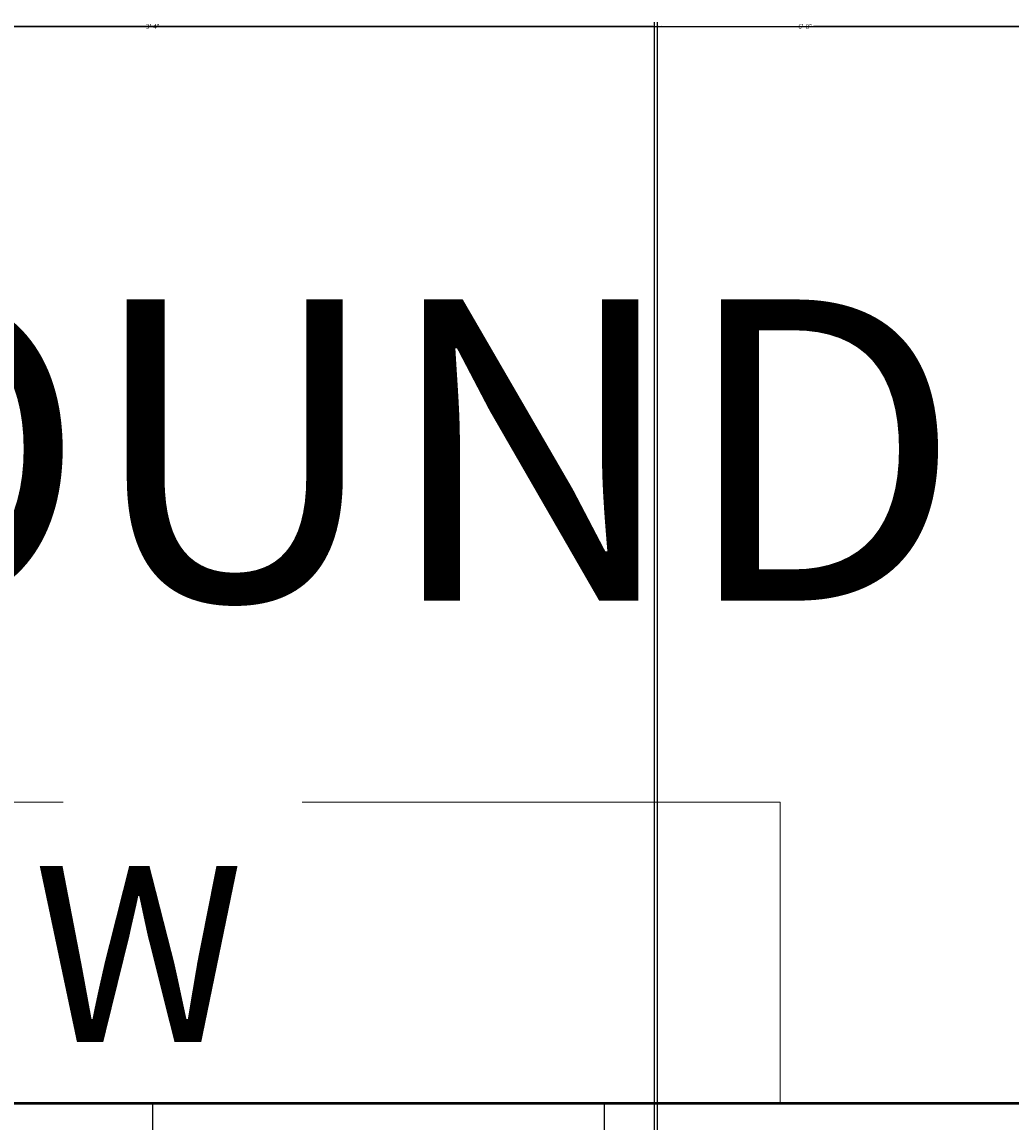
# Model space of a CAD drawing. Units: inches. Extents: x 37 to 824, y -700 to 234.
# Tile 60 of 77: x 225 to 264, y 190 to 234. Entities that reach past the tile are written whole.
import ezdxf

# ---------------------------------------------------------------- set-up
doc = ezdxf.new("R2010")
doc.units = ezdxf.units.IN
doc.header["$MEASUREMENT"] = 0
doc.linetypes.add('DASHED', pattern=[19.05, 12.7, -6.35])
for name, color, linetype, lineweight in [('A-ANNO-DIMS', 2, 'Continuous', 18), ('A-ANNO-TEXT', 7, 'Continuous', 18), ('A-GLAZ', 4, 'Continuous', 25), ('A-ROOF-OVHD', 1, 'DASHED', 18), ('A-WALL', 2, 'Continuous', 50)]:
    doc.layers.add(name, color=color, linetype=linetype, lineweight=lineweight)
doc.styles.get("Standard").update_dxf_attribs({"font": 'arial.ttf'})
doc.dimstyles.get("Standard").update_dxf_attribs({"dimtxt": 0.18, "dimasz": 0.18, "dimexe": 0.18, "dimexo": 0.0625, "dimgap": 0.09, "dimtad": 0, "dimtih": 1, "dimtoh": 1, "dimdec": 1, "dimzin": 0, "dimdsep": 46, "dimlunit": 4, "dimtxsty": 'Standard', "dimcen": 0.09, "dimadec": 0, "dimazin": 0, "dimtfac": 1, "dimtdec": 1, "dimtofl": 0, "dimtmove": 0, "dimatfit": 3, "dimfxl": 1, "dimtolj": 1, "dimtzin": 0, "dimarcsym": 0})

# ---------------------------------------------------------------- blocks, each defined once
blk = doc.blocks.new('WIN-900')
for p, q in [((0, 9), (0, 0)), ((2, 9), (2, 0)), ((20, 9), (20, 0)), ((38, 9), (38, 0)), ((40, 9), (40, 0)), ((38, 5.5), (2, 5.5)), ((38, 3.5), (2, 3.5))]:
    blk.add_line(p, q)
blk = doc.blocks.new('*D45')
at = {"layer": 'A-ANNO-DIMS', "color": 0, "lineweight": -2, "ltscale": 0.5, "transparency": 16777216}
for p, q in [((210.077, 191.153), (210.077, 234.17)), ((250.077, 191.153), (250.077, 234.17)), ((210.257, 233.99), (229.748, 233.99)), ((249.897, 233.99), (230.406, 233.99))]:
    blk.add_line(p, q, dxfattribs=at)
at = {"layer": 'A-ANNO-DIMS', "color": 0, "ltscale": 0.5, "transparency": 16777216}
for points in [[(210.257, 234.02), (210.257, 233.96), (210.077, 233.99)], [(249.897, 234.02), (249.897, 233.96), (250.077, 233.99)]]:
    blk.add_solid(points, dxfattribs=at)
at = {"layer": 'Defpoints', "color": 0, "ltscale": 0.5, "transparency": 16777216}
for p in [(250.077, 233.99), (210.077, 191.09), (250.077, 191.09)]:
    blk.add_point(p, dxfattribs=at)
at = {"layer": 'A-ANNO-DIMS', "color": 0, "ltscale": 0.5, "transparency": 16777216, "insert": (230.077, 233.99), "char_height": 0.18, "attachment_point": 5}
blk.add_mtext('\\A1;3\'-4"', dxfattribs=at)
blk = doc.blocks.new('*D46')
at = {"layer": 'A-ANNO-DIMS', "color": 0, "lineweight": -2, "ltscale": 0.5, "transparency": 16777216}
for p, q in [((250.077, 191.153), (250.077, 234.17)), ((339.077, 191.153), (339.077, 234.17)), ((250.257, 233.99), (294.249, 233.99)), ((338.897, 233.99), (294.906, 233.99))]:
    blk.add_line(p, q, dxfattribs=at)
at = {"layer": 'A-ANNO-DIMS', "color": 0, "ltscale": 0.5, "transparency": 16777216}
for points in [[(250.257, 234.02), (250.257, 233.96), (250.077, 233.99)], [(338.897, 234.02), (338.897, 233.96), (339.077, 233.99)]]:
    blk.add_solid(points, dxfattribs=at)
at = {"layer": 'Defpoints', "color": 0, "ltscale": 0.5, "transparency": 16777216}
for p in [(339.077, 233.99), (250.077, 191.09), (339.077, 191.09)]:
    blk.add_point(p, dxfattribs=at)
at = {"layer": 'A-ANNO-DIMS', "color": 0, "ltscale": 0.5, "transparency": 16777216, "insert": (294.577, 233.99), "char_height": 0.18, "attachment_point": 5}
blk.add_mtext('\\A1;7\'-5"', dxfattribs=at)
blk = doc.blocks.new('*D63')
at = {"layer": 'A-ANNO-DIMS', "color": 0, "lineweight": -2, "ltscale": 0.5, "transparency": 16777216}
for p, q in [((161.077, 191.153), (161.077, 234.17)), ((428.077, 191.153), (428.077, 234.17)), ((161.257, 233.99), (294.176, 233.99)), ((427.897, 233.99), (294.978, 233.99))]:
    blk.add_line(p, q, dxfattribs=at)
at = {"layer": 'A-ANNO-DIMS', "color": 0, "ltscale": 0.5, "transparency": 16777216}
for points in [[(161.257, 234.02), (161.257, 233.96), (161.077, 233.99)], [(427.897, 234.02), (427.897, 233.96), (428.077, 233.99)]]:
    blk.add_solid(points, dxfattribs=at)
at = {"layer": 'Defpoints', "color": 0, "ltscale": 0.5, "transparency": 16777216}
for p in [(428.077, 233.99), (161.077, 191.09), (428.077, 191.09)]:
    blk.add_point(p, dxfattribs=at)
at = {"layer": 'A-ANNO-DIMS', "color": 0, "ltscale": 0.5, "transparency": 16777216, "insert": (294.577, 233.99), "char_height": 0.18, "attachment_point": 5}
blk.add_mtext('\\A1;22\'-3"', dxfattribs=at)
blk = doc.blocks.new('*D72')
at = {"layer": 'A-ANNO-DIMS', "color": 0, "lineweight": -2, "ltscale": 0.5, "transparency": 16777216}
for p, q in [((170.077, 84.153), (170.077, 234.17)), ((250.19, 84.153), (250.19, 234.17)), ((170.257, 233.99), (209.804, 233.99)), ((250.01, 233.99), (210.463, 233.99))]:
    blk.add_line(p, q, dxfattribs=at)
at = {"layer": 'A-ANNO-DIMS', "color": 0, "ltscale": 0.5, "transparency": 16777216}
for points in [[(170.257, 234.02), (170.257, 233.96), (170.077, 233.99)], [(250.01, 234.02), (250.01, 233.96), (250.19, 233.99)]]:
    blk.add_solid(points, dxfattribs=at)
at = {"layer": 'Defpoints', "color": 0, "ltscale": 0.5, "transparency": 16777216}
for p in [(250.19, 233.99), (170.077, 84.09), (250.19, 84.09)]:
    blk.add_point(p, dxfattribs=at)
at = {"layer": 'A-ANNO-DIMS', "color": 0, "ltscale": 0.5, "transparency": 16777216, "insert": (210.133, 233.99), "char_height": 0.18, "attachment_point": 5}
blk.add_mtext('\\A1;6\'-8"', dxfattribs=at)
blk = doc.blocks.new('*D73')
at = {"layer": 'A-ANNO-DIMS', "color": 0, "lineweight": -2, "ltscale": 0.5, "transparency": 16777216}
for p, q in [((250.19, 84.153), (250.19, 234.17)), ((290.077, 81.153), (290.077, 234.17)), ((250.37, 233.99), (269.804, 233.99)), ((289.897, 233.99), (270.463, 233.99))]:
    blk.add_line(p, q, dxfattribs=at)
at = {"layer": 'A-ANNO-DIMS', "color": 0, "ltscale": 0.5, "transparency": 16777216}
for points in [[(250.37, 234.02), (250.37, 233.96), (250.19, 233.99)], [(289.897, 234.02), (289.897, 233.96), (290.077, 233.99)]]:
    blk.add_solid(points, dxfattribs=at)
at = {"layer": 'Defpoints', "color": 0, "ltscale": 0.5, "transparency": 16777216}
for p in [(290.077, 233.99), (250.19, 84.09), (290.077, 81.09)]:
    blk.add_point(p, dxfattribs=at)
at = {"layer": 'A-ANNO-DIMS', "color": 0, "ltscale": 0.5, "transparency": 16777216, "insert": (270.133, 233.99), "char_height": 0.18, "attachment_point": 5}
blk.add_mtext('\\A1;3\'-4"', dxfattribs=at)
blk = doc.blocks.new('*D87')
at = {"layer": 'A-ANNO-DIMS', "color": 0, "lineweight": -2, "ltscale": 0.5, "transparency": 16777216}
for p, q in [((216.077, -356.847), (216.077, 234.17)), ((296.077, -356.847), (296.077, 234.17)), ((216.257, 233.99), (255.747, 233.99)), ((295.897, 233.99), (256.407, 233.99))]:
    blk.add_line(p, q, dxfattribs=at)
at = {"layer": 'A-ANNO-DIMS', "color": 0, "ltscale": 0.5, "transparency": 16777216}
for points in [[(216.257, 234.02), (216.257, 233.96), (216.077, 233.99)], [(295.897, 234.02), (295.897, 233.96), (296.077, 233.99)]]:
    blk.add_solid(points, dxfattribs=at)
at = {"layer": 'Defpoints', "color": 0, "ltscale": 0.5, "transparency": 16777216}
for p in [(296.077, 233.99), (216.077, -356.91), (296.077, -356.91)]:
    blk.add_point(p, dxfattribs=at)
at = {"layer": 'A-ANNO-DIMS', "color": 0, "ltscale": 0.5, "transparency": 16777216, "insert": (256.077, 233.99), "char_height": 0.18, "attachment_point": 5}
blk.add_mtext('\\A1;6\'-8"', dxfattribs=at)

msp = doc.modelspace()

# ---------------------------------------------------------------- linework, layer by layer
at = {"layer": 'A-ROOF-OVHD', "ltscale": 1.5}
for p, q in [((255.077, 203.09), (205.077, 203.09)), ((255.077, 191.09), (255.077, 203.09)), ((250.077, 191.09), (255.077, 191.09))]:
    msp.add_line(p, q, dxfattribs=at)
at = {"layer": 'A-WALL'}
msp.add_line((161.077, 191.09), (299.077, 191.09), dxfattribs=at)

# ---------------------------------------------------------------- block references
at = {"layer": 'A-GLAZ', "rotation": 180}
msp.add_blockref('WIN-900', (250.077, 191.091), dxfattribs=at)

# ---------------------------------------------------------------- texts
at = {"layer": 'A-ANNO-TEXT'}
for s, height, p in [('GROUND  FLOOR  PLAN', 12, (193.612, 211.117)), ('W', 7, (225.324, 193.538))]:
    msp.add_text(s, height=height, dxfattribs=at).set_placement(p)

# ---------------------------------------------------------------- dimensions: what is measured, and where the dimension line sits
at = {"layer": 'A-ANNO-DIMS', "ltscale": 0.5}
for base, p1, p2, picture, middle in [((428.077, 233.99), (161.077, 191.09), (428.077, 191.09), '*D63', (294.577, 233.99)), ((250.19, 233.99), (170.077, 84.09), (250.19, 84.09), '*D72', (210.133, 233.99)), ((250.077, 233.99), (210.077, 191.09), (250.077, 191.09), '*D45', (230.077, 233.99)), ((296.077, 233.99), (216.077, -356.91), (296.077, -356.91), '*D87', (256.077, 233.99)), ((339.077, 233.99), (250.077, 191.09), (339.077, 191.09), '*D46', (294.577, 233.99)), ((290.077, 233.99), (250.19, 84.09), (290.077, 81.09), '*D73', (270.133, 233.99))]:
    dim = msp.add_linear_dim(base=base, p1=p1, p2=p2, dimstyle='Standard', override={"dimdec": 1, "dimlfac": 1, "dimrnd": 0, "dimzin": 1, "dimdsep": 46, "dimlunit": 4, "dimfrac": 2}, dxfattribs=at)
    dim.commit()
    dim.dimension.update_dxf_attribs({"geometry": picture, "text_midpoint": middle})

doc.saveas('drawing.dxf')
